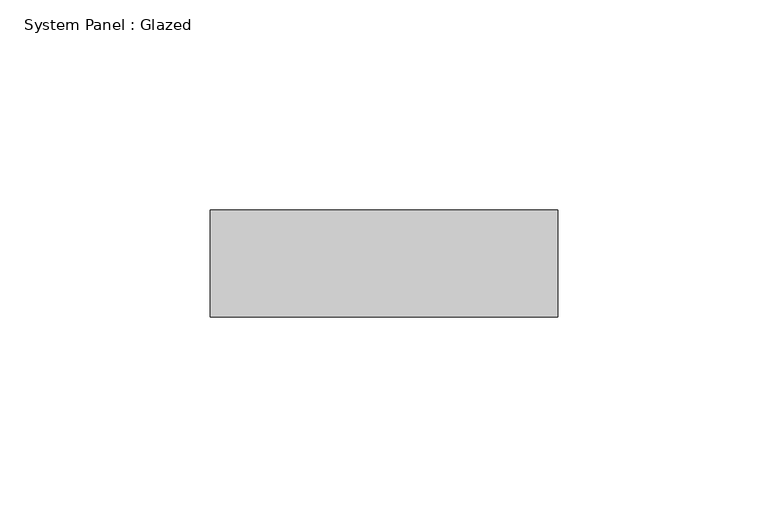
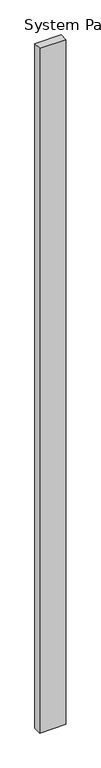
"""IFC4 building model written with IfcOpenShell, lengths in millimetres: plate geometry, System Panel : Glazed."""

from ifc_helpers import new_model, si_unit, origin, origin_with_axes, place, context, project, spatial, polyline, outline, extrude, source, transform, mapped, element, save


def system_panel_glazed_de0ba7c8(model_context):
    return source(origin(), model_context, "Body", "SweptSolid", [
        extrude(outline(polyline([(41.275, 19.05), (-41.275, 19.05), (-41.275, 44.45), (41.275, 44.45), (41.275, 19.05)])), origin_with_axes(), (0.0, 0.0, 1.0), 2287.5875),
    ])


if __name__ == "__main__":
    model = new_model("IFC4")
    model_context = context("Model", 3, world=origin())
    ifc_project = project(units=[si_unit("LENGTHUNIT", "METRE", prefix="MILLI")], contexts=[model_context])
    site = spatial("IfcSite", under=ifc_project)
    building = spatial("IfcBuilding", under=site)
    placement = place(None, origin())
    system_panel_glazed_shape = system_panel_glazed_de0ba7c8(model_context)
    element("IfcPlate", 1, ObjectType="System Panel : Glazed", at=placement, inside=building, context=model_context, shape_type="MappedRepresentation", body=[
        mapped(system_panel_glazed_shape, transform((0.0, 0.0, 0.0), x_axis=(1.0, 0.0, 0.0), y_axis=(0.0, 1.0, 0.0), z_axis=(0.0, 0.0, 1.0))),
    ])
    save(model, "model.ifc")

# Revit data of these elements
# Type "System Panel : Glazed"
#   Construction Type Id = "GSP4R"
#   Analytic Construction = "1/8 in Pilkington single glazing"
#   Visual Light Transmittance = 0.9
#   Solar Heat Gain Coefficient = 0.86
#   Heat Transfer Coefficient (U) = 1.18115 BTU/(h·ft²·°F)
#   Define Thermal Properties by = 1
# Element 1 (IfcPlate, "System Panel : Glazed")
#   Materials on its faces: "Glass"
# Materials
#   "Glass": class "Glass", colour RGB 0 128 192, transparency 0.75, Description = "Soda Lime Glass", Cost = 0
